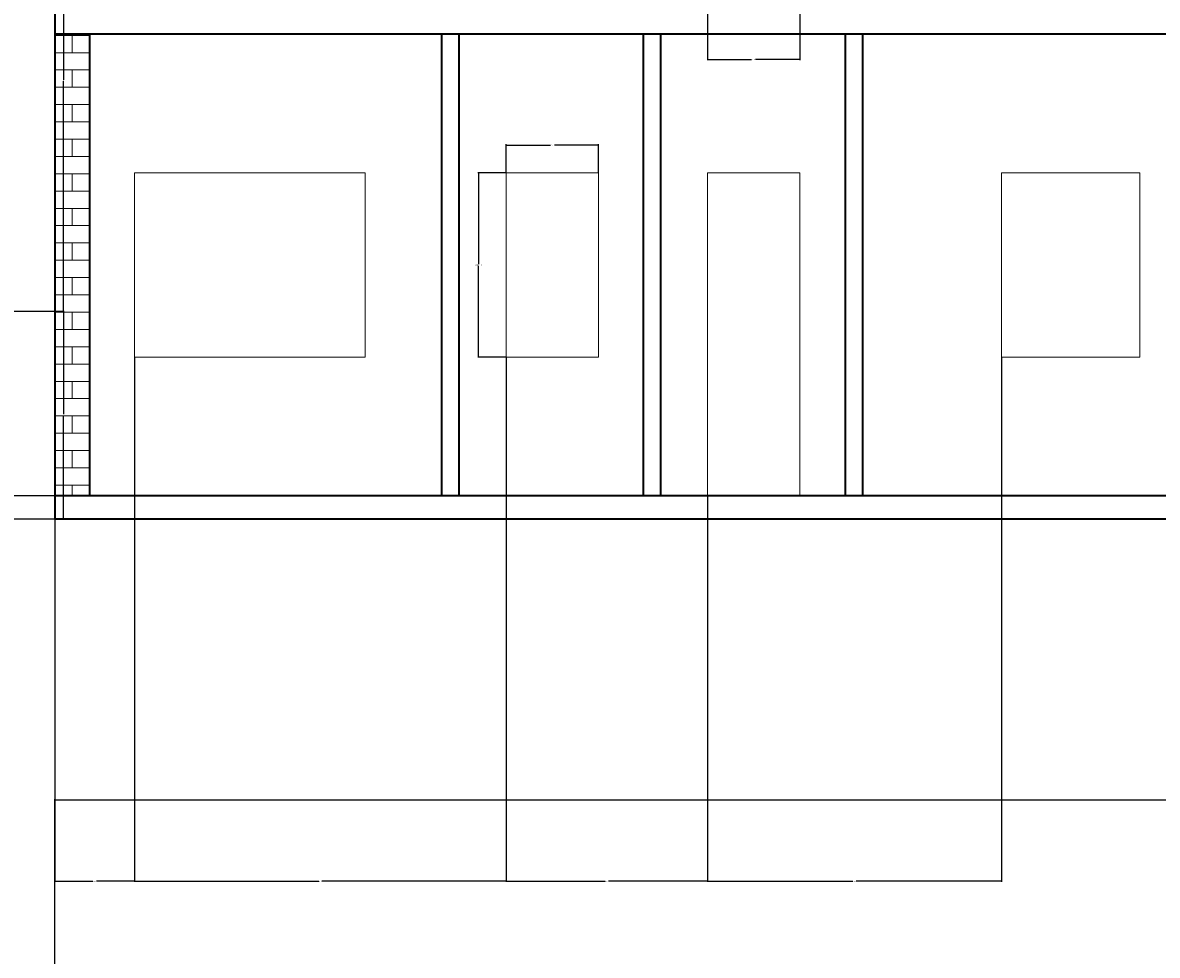
# Model space of a CAD drawing. Units: inches. Extents: x 2120 to 4013, y 1390 to 3019.
# Tile 55 of 59: x 3063 to 3358, y 2356 to 2598. Entities that reach past the tile are written whole.
import ezdxf

# ---------------------------------------------------------------- set-up
doc = ezdxf.new("R2010")
doc.units = ezdxf.units.IN
for name, color, linetype, lineweight in [('A-ANNO-DIMS', 2, 'Continuous', 18), ('A-DOOR', 3, 'Continuous', 18), ('A-GLAZ', 4, 'Continuous', 18), ('A-SECT', 7, 'Continuous', 35), ('A-WALL-PATT', 252, 'Continuous', 13)]:
    doc.layers.add(name, color=color, linetype=linetype, lineweight=lineweight)
doc.styles.get("Standard").update_dxf_attribs({"font": 'arial.ttf'})
doc.dimstyles.get("Standard").update_dxf_attribs({"dimtxt": 0.18, "dimasz": 0.18, "dimexe": 0.18, "dimexo": 0.0625, "dimgap": 0.09, "dimtad": 0, "dimtih": 1, "dimtoh": 1, "dimdec": 4, "dimzin": 0, "dimdsep": 46, "dimtxsty": 'Standard', "dimcen": 0.09, "dimadec": 0, "dimazin": 0, "dimtfac": 1, "dimtdec": 4, "dimtofl": 0, "dimtmove": 0, "dimatfit": 3, "dimfxl": 1, "dimtolj": 1, "dimtzin": 0, "dimarcsym": 0})

# ---------------------------------------------------------------- blocks, each defined once
blk = doc.blocks.new('WIN-SECT-60IN')
for p, q in [((0, 48), (0, 0)), ((60, 48), (0, 48)), ((60, 48), (60, 0)), ((60, 0), (0, 0))]:
    blk.add_line(p, q)
blk = doc.blocks.new('WIN-SECT-24IN')
for p, q in [((0, 48), (0, 0)), ((0, 48), (0, 0)), ((24, 48), (0, 48)), ((24, 48), (24, 0)), ((24, 0), (0, 0))]:
    blk.add_line(p, q)
blk = doc.blocks.new('DOOR-SECT-24IN')
for p, q in [((0, 84), (0, 0)), ((24, 84), (0, 84)), ((24, 84), (24, 0))]:
    blk.add_line(p, q)
blk = doc.blocks.new('WIN-SECT-36IN')
for p, q in [((0, 48), (0, 0)), ((36, 48), (0, 48)), ((36, 48), (36, 0)), ((36, 0), (0, 0))]:
    blk.add_line(p, q)
blk = doc.blocks.new('*D201')
at = {"layer": 'A-ANNO-DIMS', "color": 0, "lineweight": -2, "transparency": 16777216}
for p, q in [((3189.03, 2559.31), (3181.72, 2559.31)), ((3181.9, 2559.13), (3181.9, 2535.49)), ((3181.9, 2511.49), (3181.9, 2535.13)), ((3189.03, 2511.31), (3181.72, 2511.31))]:
    blk.add_line(p, q, dxfattribs=at)
at = {"layer": 'A-ANNO-DIMS', "color": 0, "transparency": 16777216}
for points in [[(3181.87, 2559.13), (3181.93, 2559.13), (3181.9, 2559.31)], [(3181.87, 2511.49), (3181.93, 2511.49), (3181.9, 2511.31)]]:
    blk.add_solid(points, dxfattribs=at)
at = {"layer": 'Defpoints', "color": 0, "transparency": 16777216}
for p in [(3181.9, 2559.31), (3189.1, 2559.31), (3189.1, 2511.31)]:
    blk.add_point(p, dxfattribs=at)
at = {"layer": 'A-ANNO-DIMS', "color": 0, "transparency": 16777216, "insert": (3181.9, 2535.31), "char_height": 0.18, "attachment_point": 5}
blk.add_mtext('\\A1;WINDOW 48 TYP.', dxfattribs=at)
blk = doc.blocks.new('*D202')
at = {"layer": 'A-ANNO-DIMS', "color": 0, "lineweight": -2, "transparency": 16777216}
for p, q in [((3189.1, 2559.37), (3189.1, 2566.69)), ((3189.28, 2566.51), (3200.57, 2566.51)), ((3212.92, 2566.51), (3201.63, 2566.51)), ((3213.1, 2559.37), (3213.1, 2566.69))]:
    blk.add_line(p, q, dxfattribs=at)
at = {"layer": 'A-ANNO-DIMS', "color": 0, "transparency": 16777216}
for points in [[(3189.28, 2566.54), (3189.28, 2566.48), (3189.1, 2566.51)], [(3212.92, 2566.54), (3212.92, 2566.48), (3213.1, 2566.51)]]:
    blk.add_solid(points, dxfattribs=at)
at = {"layer": 'Defpoints', "color": 0, "transparency": 16777216}
for p in [(3213.1, 2566.51), (3189.1, 2559.31), (3213.1, 2559.31)]:
    blk.add_point(p, dxfattribs=at)
at = {"layer": 'A-ANNO-DIMS', "color": 0, "transparency": 16777216, "insert": (3201.1, 2566.51), "char_height": 0.18, "attachment_point": 5}
blk.add_mtext('\\A1;24 TYP.', dxfattribs=at)
blk = doc.blocks.new('*D204')
at = {"layer": 'A-ANNO-DIMS', "color": 0, "lineweight": -2, "transparency": 16777216}
for p, q in [((3241.44, 2601.25), (3241.44, 2588.53)), ((3265.44, 2601.25), (3265.44, 2588.53)), ((3241.62, 2588.71), (3252.91, 2588.71)), ((3265.26, 2588.71), (3253.97, 2588.71))]:
    blk.add_line(p, q, dxfattribs=at)
at = {"layer": 'A-ANNO-DIMS', "color": 0, "transparency": 16777216}
for points in [[(3241.62, 2588.74), (3241.62, 2588.68), (3241.44, 2588.71)], [(3265.26, 2588.74), (3265.26, 2588.68), (3265.44, 2588.71)]]:
    blk.add_solid(points, dxfattribs=at)
at = {"layer": 'Defpoints', "color": 0, "transparency": 16777216}
for p in [(3241.44, 2601.31), (3265.44, 2601.31), (3265.44, 2588.71)]:
    blk.add_point(p, dxfattribs=at)
at = {"layer": 'A-ANNO-DIMS', "color": 0, "transparency": 16777216, "insert": (3253.44, 2588.71), "char_height": 0.18, "attachment_point": 5}
blk.add_mtext('\\A1;24 TYP.', dxfattribs=at)
blk = doc.blocks.new('*D216')
at = {"layer": 'A-ANNO-DIMS', "color": 0, "lineweight": -2, "transparency": 16777216}
for p, q in [((3071.73, 2352.59), (3071.73, 2396.46)), ((3071.91, 2396.28), (3444.95, 2396.28)), ((3818.55, 2396.28), (3445.52, 2396.28)), ((3818.73, 2352.59), (3818.73, 2396.46))]:
    blk.add_line(p, q, dxfattribs=at)
at = {"layer": 'A-ANNO-DIMS', "color": 0, "transparency": 16777216}
for points in [[(3071.91, 2396.31), (3071.91, 2396.25), (3071.73, 2396.28)], [(3818.55, 2396.31), (3818.55, 2396.25), (3818.73, 2396.28)]]:
    blk.add_solid(points, dxfattribs=at)
at = {"layer": 'Defpoints', "color": 0, "transparency": 16777216}
for p in [(3818.73, 2396.28), (3071.73, 2352.53), (3818.73, 2352.53)]:
    blk.add_point(p, dxfattribs=at)
at = {"layer": 'A-ANNO-DIMS', "color": 0, "transparency": 16777216, "insert": (3445.23, 2396.28), "char_height": 0.18, "attachment_point": 5}
blk.add_mtext('\\A1;747', dxfattribs=at)
blk = doc.blocks.new('*D233')
at = {"layer": 'A-ANNO-DIMS', "color": 0, "lineweight": -2, "transparency": 16777216}
for p, q in [((3009.8, 2523.31), (3074.11, 2523.31)), ((3073.93, 2523.13), (3073.93, 2496.49)), ((3073.93, 2469.49), (3073.93, 2496.13)), ((3009.8, 2469.31), (3074.11, 2469.31))]:
    blk.add_line(p, q, dxfattribs=at)
at = {"layer": 'A-ANNO-DIMS', "color": 0, "transparency": 16777216}
for points in [[(3073.9, 2523.13), (3073.96, 2523.13), (3073.93, 2523.31)], [(3073.9, 2469.49), (3073.96, 2469.49), (3073.93, 2469.31)]]:
    blk.add_solid(points, dxfattribs=at)
at = {"layer": 'Defpoints', "color": 0, "transparency": 16777216}
for p in [(3009.73, 2523.31), (3073.93, 2523.31), (3009.73, 2469.31)]:
    blk.add_point(p, dxfattribs=at)
at = {"layer": 'A-ANNO-DIMS', "color": 0, "transparency": 16777216, "insert": (3073.93, 2496.31), "char_height": 0.18, "attachment_point": 5}
blk.add_mtext('\\A1;54', dxfattribs=at)
blk = doc.blocks.new('*D234')
at = {"layer": 'A-ANNO-DIMS', "color": 0, "lineweight": -2, "transparency": 16777216}
for p, q in [((3033.8, 2643.31), (3074.11, 2643.31)), ((3073.93, 2643.13), (3073.93, 2583.49)), ((3073.93, 2523.49), (3073.93, 2583.13)), ((3009.8, 2523.31), (3074.11, 2523.31))]:
    blk.add_line(p, q, dxfattribs=at)
at = {"layer": 'A-ANNO-DIMS', "color": 0, "transparency": 16777216}
for points in [[(3073.9, 2643.13), (3073.96, 2643.13), (3073.93, 2643.31)], [(3073.9, 2523.49), (3073.96, 2523.49), (3073.93, 2523.31)]]:
    blk.add_solid(points, dxfattribs=at)
at = {"layer": 'Defpoints', "color": 0, "transparency": 16777216}
for p in [(3033.73, 2643.31), (3073.93, 2643.31), (3009.73, 2523.31)]:
    blk.add_point(p, dxfattribs=at)
at = {"layer": 'A-ANNO-DIMS', "color": 0, "transparency": 16777216, "insert": (3073.93, 2583.31), "char_height": 0.18, "attachment_point": 5}
blk.add_mtext('\\A1;120', dxfattribs=at)
blk = doc.blocks.new('*D238')
at = {"layer": 'A-ANNO-DIMS', "color": 0, "lineweight": -2, "transparency": 16777216}
for p, q in [((3071.67, 2601.31), (3026.6, 2601.31)), ((3026.78, 2601.13), (3026.78, 2538.49)), ((3026.78, 2475.49), (3026.78, 2538.13)), ((3071.67, 2475.31), (3026.6, 2475.31))]:
    blk.add_line(p, q, dxfattribs=at)
at = {"layer": 'A-ANNO-DIMS', "color": 0, "transparency": 16777216}
for points in [[(3026.75, 2601.13), (3026.81, 2601.13), (3026.78, 2601.31)], [(3026.75, 2475.49), (3026.81, 2475.49), (3026.78, 2475.31)]]:
    blk.add_solid(points, dxfattribs=at)
at = {"layer": 'Defpoints', "color": 0, "transparency": 16777216}
for p in [(3026.78, 2601.31), (3071.73, 2601.31), (3071.73, 2475.31)]:
    blk.add_point(p, dxfattribs=at)
at = {"layer": 'A-ANNO-DIMS', "color": 0, "transparency": 16777216, "insert": (3026.78, 2538.31), "char_height": 0.18, "attachment_point": 5}
blk.add_mtext('\\A1;126', dxfattribs=at)
blk = doc.blocks.new('*D241')
at = {"layer": 'A-ANNO-DIMS', "color": 0, "lineweight": -2, "transparency": 16777216}
for p, q in [((3092.38, 2511.25), (3092.38, 2374.91)), ((3071.73, 2475.25), (3071.73, 2374.91)), ((3071.91, 2375.09), (3081.59, 2375.09)), ((3092.2, 2375.09), (3082.52, 2375.09))]:
    blk.add_line(p, q, dxfattribs=at)
at = {"layer": 'A-ANNO-DIMS', "color": 0, "transparency": 16777216}
for points in [[(3071.91, 2375.12), (3071.91, 2375.06), (3071.73, 2375.09)], [(3092.2, 2375.12), (3092.2, 2375.06), (3092.38, 2375.09)]]:
    blk.add_solid(points, dxfattribs=at)
at = {"layer": 'Defpoints', "color": 0, "transparency": 16777216}
for p in [(3092.38, 2511.31), (3071.73, 2475.31), (3092.38, 2375.09)]:
    blk.add_point(p, dxfattribs=at)
at = {"layer": 'A-ANNO-DIMS', "color": 0, "transparency": 16777216, "insert": (3082.06, 2375.09), "char_height": 0.18, "attachment_point": 5}
blk.add_mtext('\\A1;20.646', dxfattribs=at)
blk = doc.blocks.new('*D242')
at = {"layer": 'A-ANNO-DIMS', "color": 0, "lineweight": -2, "transparency": 16777216}
for p, q in [((3092.38, 2511.25), (3092.38, 2374.91)), ((3189.1, 2511.25), (3189.1, 2374.91)), ((3092.56, 2375.09), (3140.35, 2375.09)), ((3188.92, 2375.09), (3141.13, 2375.09))]:
    blk.add_line(p, q, dxfattribs=at)
at = {"layer": 'A-ANNO-DIMS', "color": 0, "transparency": 16777216}
for points in [[(3092.56, 2375.12), (3092.56, 2375.06), (3092.38, 2375.09)], [(3188.92, 2375.12), (3188.92, 2375.06), (3189.1, 2375.09)]]:
    blk.add_solid(points, dxfattribs=at)
at = {"layer": 'Defpoints', "color": 0, "transparency": 16777216}
for p in [(3092.38, 2511.31), (3189.1, 2511.31), (3189.1, 2375.09)]:
    blk.add_point(p, dxfattribs=at)
at = {"layer": 'A-ANNO-DIMS', "color": 0, "transparency": 16777216, "insert": (3140.74, 2375.09), "char_height": 0.18, "attachment_point": 5}
blk.add_mtext('\\A1;96.72', dxfattribs=at)
blk = doc.blocks.new('*D243')
at = {"layer": 'A-ANNO-DIMS', "color": 0, "lineweight": -2, "transparency": 16777216}
for p, q in [((3189.1, 2511.25), (3189.1, 2374.91)), ((3241.44, 2475.25), (3241.44, 2374.91)), ((3189.28, 2375.09), (3214.87, 2375.09)), ((3241.26, 2375.09), (3215.66, 2375.09))]:
    blk.add_line(p, q, dxfattribs=at)
at = {"layer": 'A-ANNO-DIMS', "color": 0, "transparency": 16777216}
for points in [[(3189.28, 2375.12), (3189.28, 2375.06), (3189.1, 2375.09)], [(3241.26, 2375.12), (3241.26, 2375.06), (3241.44, 2375.09)]]:
    blk.add_solid(points, dxfattribs=at)
at = {"layer": 'Defpoints', "color": 0, "transparency": 16777216}
for p in [(3189.1, 2511.31), (3241.44, 2475.31), (3241.44, 2375.09)]:
    blk.add_point(p, dxfattribs=at)
at = {"layer": 'A-ANNO-DIMS', "color": 0, "transparency": 16777216, "insert": (3215.27, 2375.09), "char_height": 0.18, "attachment_point": 5}
blk.add_mtext('\\A1;52.34', dxfattribs=at)
blk = doc.blocks.new('*D244')
at = {"layer": 'A-ANNO-DIMS', "color": 0, "lineweight": -2, "transparency": 16777216}
for p, q in [((3317.91, 2511.25), (3317.91, 2374.91)), ((3241.44, 2475.25), (3241.44, 2374.91)), ((3241.62, 2375.09), (3279.28, 2375.09)), ((3317.73, 2375.09), (3280.07, 2375.09))]:
    blk.add_line(p, q, dxfattribs=at)
at = {"layer": 'A-ANNO-DIMS', "color": 0, "transparency": 16777216}
for points in [[(3241.62, 2375.12), (3241.62, 2375.06), (3241.44, 2375.09)], [(3317.73, 2375.12), (3317.73, 2375.06), (3317.91, 2375.09)]]:
    blk.add_solid(points, dxfattribs=at)
at = {"layer": 'Defpoints', "color": 0, "transparency": 16777216}
for p in [(3317.91, 2511.31), (3241.44, 2475.31), (3317.91, 2375.09)]:
    blk.add_point(p, dxfattribs=at)
at = {"layer": 'A-ANNO-DIMS', "color": 0, "transparency": 16777216, "insert": (3279.67, 2375.09), "char_height": 0.18, "attachment_point": 5}
blk.add_mtext('\\A1;76.48', dxfattribs=at)

msp = doc.modelspace()

# ---------------------------------------------------------------- hatches: boundary and pattern name
at = {"layer": 'A-WALL-PATT'}
h = msp.add_hatch(dxfattribs=at)
h.set_pattern_fill('ANSI32', color=256)
h.paths.add_polyline_path([(2271.7331, 2343.531), (2283.3788, 2343.531), (2283.3788, 2348.031), (2283.3788, 2352.5306), (2262.7331, 2352.5306), (2262.7331, 2182.638), (2267.2331, 2182.638), (2271.7331, 2182.638), (2271.7331, 2219.031), (2391.7331, 2219.031), (2391.7331, 2214.189), (2393.9831, 2214.189), (2396.2331, 2214.189), (2396.2331, 2219.031), (2420.2331, 2219.031), (2420.2331, 2225.7535), (2417.2197, 2225.7535), (2415.7331, 2225.7535), (2415.7331, 2223.5306), (2271.7331, 2223.5306)])
h.paths.add_polyline_path([(2380.0942, 2352.5306), (2343.3788, 2352.5306), (2343.3788, 2343.531), (2363.2331, 2343.531), (2363.2331, 2288.8489), (2365.4831, 2288.8489), (2367.7331, 2288.8489), (2367.7331, 2343.531), (2380.0942, 2343.531)], flags=17)
h.paths.add_polyline_path([(2432.4339, 2352.5306), (2404.0943, 2352.5306), (2404.0943, 2343.531), (2415.7331, 2343.531), (2415.7331, 2264.0306), (2367.7331, 2264.0306), (2367.7331, 2266.4872), (2363.2331, 2266.4872), (2363.2331, 2259.531), (2367.7331, 2259.531), (2415.7331, 2259.531), (2415.7331, 2255.0658), (2420.2331, 2255.0658), (2420.2331, 2259.531), (2424.5717, 2259.531), (2424.5717, 2261.781), (2424.5717, 2264.0306), (2420.2331, 2264.0306), (2420.2331, 2343.531), (2432.4339, 2343.531)])
h.paths.add_polyline_path([(2508.9115, 2352.5306), (2456.4339, 2352.5306), (2456.4339, 2343.531), (2468.2331, 2343.531), (2468.2331, 2264.0306), (2448.0487, 2264.0306), (2448.0487, 2259.531), (2468.2331, 2259.531), (2468.2331, 2255.5496), (2472.7331, 2255.5496), (2472.7331, 2343.531), (2508.9115, 2343.531)])
h.paths.add_polyline_path([(2637.7331, 2352.5306), (2544.9116, 2352.5306), (2544.9116, 2343.531), (2589.7331, 2343.531), (2633.2331, 2343.531), (2637.7331, 2343.531)])
h.paths.add_polyline_path([(2594.2331, 2343.5306), (2589.7331, 2343.5306), (2589.7331, 2259.5306), (2589.7331, 2252.4915), (2591.9831, 2252.4915), (2594.2331, 2252.4915)])
h.paths.add_polyline_path([(2637.7331, 2223.5306), (2594.2331, 2223.5306), (2594.2331, 2230.1988), (2591.9831, 2230.1988), (2589.7331, 2230.1988), (2589.7331, 2223.5306), (2472.7331, 2223.5306), (2468.2331, 2223.5306), (2468.2331, 2219.031), (2628.7331, 2219.031), (2628.7331, 2138.031), (2637.7331, 2138.031)])
h.paths.add_polyline_path([(3822.6535, 2458.4402), (3874.9468, 2458.4402), (3874.9468, 2476.9866), (3822.6535, 2476.9866)], flags=9)
h.paths.add_polyline_path([(3834.6921, 2781.8174), (3935.9206, 2781.8174), (3935.9206, 2800.3638), (3834.6921, 2800.3638)], flags=9)
h.paths.add_polyline_path([(3832.2843, 2837.9683), (3884.5776, 2837.9683), (3884.5776, 2856.5146), (3832.2843, 2856.5146)], flags=9)
h.paths.add_polyline_path([(3830.9388, 2861.4782), (3956.8958, 2861.4782), (3956.8958, 2880.0245), (3830.9388, 2880.0245)], flags=9)
h.paths.add_polyline_path([(3870.6966, 2352.5752), (3887.9272, 2352.5752), (3887.9272, 2377.3037), (3870.6966, 2377.3037)], flags=9)
h.paths.add_polyline_path([(3289.2701, 2413.161), (3435.2223, 2413.161), (3435.2223, 2450.2538), (3289.2701, 2450.2538)], flags=9)
h.paths.add_polyline_path([(2487.6944, 2414.3601), (2637.8335, 2414.3601), (2637.8335, 2451.4528), (2487.6944, 2451.4528)], flags=9)
h.paths.add_polyline_path([(2567.3724, 1457.9199), (2815.296, 1457.9199), (2815.296, 1495.0127), (2567.3724, 1495.0127)], flags=9)
h.paths.add_polyline_path([(2655.3825, 2093.2363), (2685.9555, 2093.2363), (2685.9555, 2111.8937), (2655.3825, 2111.8937)], flags=9)
h.paths.add_polyline_path([(2543.9218, 1550.6671), (2587.8406, 1550.6671), (2587.8406, 1569.3244), (2543.9218, 1569.3244)], flags=9)
h.paths.add_polyline_path([(2905.1384, 1543.8113), (2949.0572, 1543.8113), (2949.0572, 1562.4686), (2905.1384, 1562.4686)], flags=9)
h.paths.add_polyline_path([(2736.4118, 1702.4736), (2784.2153, 1702.4736), (2784.2153, 1721.1309), (2736.4118, 1721.1309)], flags=9)
h.paths.add_polyline_path([(2912.8666, 1710.4168), (2951.707, 1710.4168), (2951.707, 1729.0741), (2912.8666, 1729.0741)], flags=9)
h.paths.add_polyline_path([(2923.5785, 1763.5038), (2959.7279, 1763.5038), (2959.7279, 1782.1611), (2923.5785, 1782.1611)], flags=9)
h.paths.add_polyline_path([(2925.2114, 1809.6137), (2967.1861, 1809.6137), (2967.1861, 1828.271), (2925.2114, 1828.271)], flags=9)
h.paths.add_polyline_path([(2996.2711, 1878.9003), (2996.2711, 1913.109), (2977.6138, 1913.109), (2977.6138, 1878.9003)], flags=9)
h.paths.add_polyline_path([(2883.0859, 1895.7192), (2927.1855, 1895.7192), (2927.1855, 1914.3766), (2883.0859, 1914.3766)], flags=9)
h.paths.add_polyline_path([(2787.3924, 1810.8013), (2841.0213, 1810.8013), (2841.0213, 1829.4587), (2787.3924, 1829.4587)], flags=9)
h.paths.add_polyline_path([(2775.6399, 2101.7395), (2829.2689, 2101.7395), (2829.2689, 2120.3968), (2775.6399, 2120.3968)], flags=9)
h.paths.add_polyline_path([(2913.0263, 2075.817), (2951.8667, 2075.817), (2951.8667, 2094.4744), (2913.0263, 2094.4744)], flags=9)
h.paths.add_polyline_path([(2929.966, 2133.3669), (2966.1154, 2133.3669), (2966.1154, 2152.0243), (2929.966, 2152.0243)], flags=9)
h.paths.add_polyline_path([(2932.7502, 2182.6088), (2968.8996, 2182.6088), (2968.8996, 2201.2662), (2932.7502, 2201.2662)], flags=9)
h.paths.add_polyline_path([(2996.0681, 2266.3173), (2996.0681, 2300.5261), (2977.4108, 2300.5261), (2977.4108, 2266.3173)], flags=9)
h.paths.add_polyline_path([(2885.1039, 2279.2186), (2929.2035, 2279.2186), (2929.2035, 2297.8759), (2885.1039, 2297.8759)], flags=9)
h.paths.add_polyline_path([(2735.7042, 2218.3197), (2783.5078, 2218.3197), (2783.5078, 2236.9771), (2735.7042, 2236.9771)], flags=9)
h.paths.add_polyline_path([(2635.6049, 2044.0085), (2648.9678, 2044.0085), (2648.9678, 2054.312), (2635.6049, 2054.312)], flags=9)
h.paths.add_polyline_path([(2714.0148, 1923.0473), (2727.3777, 1923.0473), (2727.3777, 1933.3508), (2714.0148, 1933.3508)], flags=9)
h.paths.add_polyline_path([(2709.0345, 1988.1628), (2722.3974, 1988.1628), (2722.3974, 1998.4663), (2709.0345, 1998.4663)], flags=9)
h.paths.add_polyline_path([(2592.8935, 1962.1763), (2606.2564, 1962.1763), (2606.2564, 1972.4799), (2592.8935, 1972.4799)], flags=9)
h.paths.add_polyline_path([(2618.3996, 1985.9724), (2644.1942, 1985.9724), (2644.1942, 1996.2759), (2618.3996, 1996.2759)], flags=9)
h.paths.add_polyline_path([(2601.279, 1920.5869), (2614.6419, 1920.5869), (2614.6419, 1930.8904), (2601.279, 1930.8904)], flags=9)
h.paths.add_polyline_path([(2692.3278, 1932.7645), (2704.5311, 1932.7645), (2704.5311, 1943.0681), (2692.3278, 1943.0681)], flags=9)
h.paths.add_polyline_path([(2311.122, 1672.7318), (2355.0408, 1672.7318), (2355.0408, 1691.3892), (2311.122, 1691.3892)], flags=9)
h.paths.add_polyline_path([(2456.2551, 1632.3198), (2492.4796, 1632.3198), (2492.4796, 1650.9772), (2456.2551, 1650.9772)], flags=9)
h.paths.add_polyline_path([(2401.0766, 1631.4793), (2437.301, 1631.4793), (2437.301, 1650.1367), (2401.0766, 1650.1367)], flags=9)
h.paths.add_polyline_path([(2546.7054, 1700.9235), (2594.509, 1700.9235), (2594.509, 1719.5809), (2546.7054, 1719.5809)], flags=9)
h.paths.add_polyline_path([(2445.4866, 1766.9937), (2497.5261, 1766.9937), (2497.5261, 1785.651), (2445.4866, 1785.651)], flags=9)
h.paths.add_polyline_path([(2287.9992, 1739.7675), (2326.8396, 1739.7675), (2326.8396, 1758.4248), (2287.9992, 1758.4248)], flags=9)
h.paths.add_polyline_path([(2458.5279, 1924.7607), (2510.5675, 1924.7607), (2510.5675, 1943.4181), (2458.5279, 1943.4181)], flags=9)
h.paths.add_polyline_path([(2309.2811, 1902.7642), (2345.4305, 1902.7642), (2345.4305, 1921.4215), (2309.2811, 1921.4215)], flags=9)
h.paths.add_polyline_path([(2490.7554, 2018.9392), (2530.7896, 2018.9392), (2530.7896, 2037.5965), (2490.7554, 2037.5965)], flags=9)
h.paths.add_polyline_path([(2402.143, 2024.7393), (2438.5414, 2024.7393), (2438.5414, 2043.3966), (2402.143, 2043.3966)], flags=9)
h.paths.add_polyline_path([(2287.856, 1931.7926), (2326.6964, 1931.7926), (2326.6964, 1950.4499), (2287.856, 1950.4499)], flags=9)
h.paths.add_polyline_path([(2281.7979, 2193.5771), (2320.6383, 2193.5771), (2320.6383, 2212.2344), (2281.7979, 2212.2344)], flags=25)
h.paths.add_polyline_path([(2484.0754, 2093.892), (2536.115, 2093.892), (2536.115, 2112.5494), (2484.0754, 2112.5494)], flags=9)
h.paths.add_polyline_path([(2624.7948, 2281.8639), (2624.7948, 2311.4137), (2606.1375, 2311.4137), (2606.1375, 2281.8639)], flags=9)
h.paths.add_polyline_path([(2507.5036, 2290.3639), (2541.934, 2290.3639), (2541.934, 2309.0212), (2507.5036, 2309.0212)], flags=9)
h.paths.add_polyline_path([(2423.1076, 2285.2202), (2459.332, 2285.2202), (2459.332, 2303.8776), (2423.1076, 2303.8776)], flags=9)
h.paths.add_polyline_path([(2374.5467, 2289.6272), (2410.7711, 2289.6272), (2410.7711, 2308.2846), (2374.5467, 2308.2846)], flags=25)
h.paths.add_polyline_path([(2277.4907, 2227.5651), (2316.3311, 2227.5651), (2316.3311, 2246.2224), (2277.4907, 2246.2224)], flags=25)
h.paths.add_polyline_path([(2655.3825, 2093.2367), (2685.9555, 2093.2367), (2685.9555, 2111.894), (2655.3825, 2111.894)], flags=9)
h.paths.add_polyline_path([(2543.9217, 1550.6674), (2587.8406, 1550.6674), (2587.8406, 1569.3247), (2543.9217, 1569.3247)], flags=9)
h.paths.add_polyline_path([(2905.1384, 1543.8116), (2949.0572, 1543.8116), (2949.0572, 1562.4689), (2905.1384, 1562.4689)], flags=9)
h.paths.add_polyline_path([(2736.4118, 1702.4739), (2784.2153, 1702.4739), (2784.2153, 1721.1312), (2736.4118, 1721.1312)], flags=9)
h.paths.add_polyline_path([(2912.8666, 1710.4171), (2951.707, 1710.4171), (2951.707, 1729.0744), (2912.8666, 1729.0744)], flags=9)
h.paths.add_polyline_path([(2923.5785, 1763.5041), (2959.7279, 1763.5041), (2959.7279, 1782.1614), (2923.5785, 1782.1614)], flags=9)
h.paths.add_polyline_path([(2925.2114, 1809.614), (2967.1861, 1809.614), (2967.1861, 1828.2713), (2925.2114, 1828.2713)], flags=9)
h.paths.add_polyline_path([(2996.2711, 1878.9006), (2996.2711, 1913.1094), (2977.6137, 1913.1094), (2977.6137, 1878.9006)], flags=9)
h.paths.add_polyline_path([(2883.0859, 1895.7195), (2927.1855, 1895.7195), (2927.1855, 1914.3769), (2883.0859, 1914.3769)], flags=9)
h.paths.add_polyline_path([(2787.3924, 1810.8016), (2841.0213, 1810.8016), (2841.0213, 1829.459), (2787.3924, 1829.459)], flags=9)
h.paths.add_polyline_path([(2775.6399, 2101.7398), (2829.2688, 2101.7398), (2829.2688, 2120.3971), (2775.6399, 2120.3971)], flags=9)
h.paths.add_polyline_path([(2913.0263, 2075.8173), (2951.8667, 2075.8173), (2951.8667, 2094.4747), (2913.0263, 2094.4747)], flags=9)
h.paths.add_polyline_path([(2929.966, 2133.3672), (2966.1154, 2133.3672), (2966.1154, 2152.0246), (2929.966, 2152.0246)], flags=9)
h.paths.add_polyline_path([(2932.7502, 2182.6091), (2968.8996, 2182.6091), (2968.8996, 2201.2665), (2932.7502, 2201.2665)], flags=9)
h.paths.add_polyline_path([(2996.0681, 2266.3176), (2996.0681, 2300.5264), (2977.4108, 2300.5264), (2977.4108, 2266.3176)], flags=9)
h.paths.add_polyline_path([(2885.1039, 2279.2189), (2929.2035, 2279.2189), (2929.2035, 2297.8762), (2885.1039, 2297.8762)], flags=9)
h.paths.add_polyline_path([(2735.7042, 2218.32), (2783.5078, 2218.32), (2783.5078, 2236.9774), (2735.7042, 2236.9774)], flags=9)
h.paths.add_polyline_path([(2635.6048, 2044.0088), (2648.9677, 2044.0088), (2648.9677, 2054.3123), (2635.6048, 2054.3123)], flags=9)
h.paths.add_polyline_path([(2714.0148, 1923.0476), (2727.3777, 1923.0476), (2727.3777, 1933.3511), (2714.0148, 1933.3511)], flags=9)
h.paths.add_polyline_path([(2709.0345, 1988.1631), (2722.3974, 1988.1631), (2722.3974, 1998.4666), (2709.0345, 1998.4666)], flags=9)
h.paths.add_polyline_path([(2592.8935, 1962.1766), (2606.2564, 1962.1766), (2606.2564, 1972.4802), (2592.8935, 1972.4802)], flags=9)
h.paths.add_polyline_path([(2618.3995, 1985.9727), (2644.1942, 1985.9727), (2644.1942, 1996.2762), (2618.3995, 1996.2762)], flags=9)
h.paths.add_polyline_path([(2601.279, 1920.5872), (2614.6419, 1920.5872), (2614.6419, 1930.8908), (2601.279, 1930.8908)], flags=9)
h.paths.add_polyline_path([(2692.3278, 1932.7648), (2704.5311, 1932.7648), (2704.5311, 1943.0684), (2692.3278, 1943.0684)], flags=9)
h.paths.add_polyline_path([(2311.122, 1672.7321), (2355.0408, 1672.7321), (2355.0408, 1691.3895), (2311.122, 1691.3895)], flags=9)
h.paths.add_polyline_path([(2456.2551, 1632.3201), (2492.4795, 1632.3201), (2492.4795, 1650.9775), (2456.2551, 1650.9775)], flags=9)
h.paths.add_polyline_path([(2401.0766, 1631.4796), (2437.301, 1631.4796), (2437.301, 1650.137), (2401.0766, 1650.137)], flags=9)
h.paths.add_polyline_path([(2546.7054, 1700.9238), (2594.509, 1700.9238), (2594.509, 1719.5812), (2546.7054, 1719.5812)], flags=9)
h.paths.add_polyline_path([(2445.4866, 1766.994), (2497.5261, 1766.994), (2497.5261, 1785.6513), (2445.4866, 1785.6513)], flags=9)
h.paths.add_polyline_path([(2287.9992, 1739.7678), (2326.8396, 1739.7678), (2326.8396, 1758.4251), (2287.9992, 1758.4251)], flags=9)
h.paths.add_polyline_path([(2458.5279, 1924.7611), (2510.5675, 1924.7611), (2510.5675, 1943.4184), (2458.5279, 1943.4184)], flags=9)
h.paths.add_polyline_path([(2309.2811, 1902.7645), (2345.4305, 1902.7645), (2345.4305, 1921.4218), (2309.2811, 1921.4218)], flags=9)
h.paths.add_polyline_path([(2490.7554, 2018.9395), (2530.7895, 2018.9395), (2530.7895, 2037.5968), (2490.7554, 2037.5968)], flags=9)
h.paths.add_polyline_path([(2402.143, 2024.7396), (2438.5413, 2024.7396), (2438.5413, 2043.3969), (2402.143, 2043.3969)], flags=9)
h.paths.add_polyline_path([(2287.856, 1931.7929), (2326.6964, 1931.7929), (2326.6964, 1950.4502), (2287.856, 1950.4502)], flags=9)
h.paths.add_polyline_path([(2281.7979, 2193.5774), (2320.6383, 2193.5774), (2320.6383, 2212.2347), (2281.7979, 2212.2347)], flags=25)
h.paths.add_polyline_path([(2484.0754, 2093.8924), (2536.115, 2093.8924), (2536.115, 2112.5497), (2484.0754, 2112.5497)], flags=9)
h.paths.add_polyline_path([(2624.7948, 2281.8642), (2624.7948, 2311.414), (2606.1374, 2311.414), (2606.1374, 2281.8642)], flags=9)
h.paths.add_polyline_path([(2507.5035, 2290.3642), (2541.934, 2290.3642), (2541.934, 2309.0215), (2507.5035, 2309.0215)], flags=9)
h.paths.add_polyline_path([(2423.1075, 2285.2205), (2459.332, 2285.2205), (2459.332, 2303.8779), (2423.1075, 2303.8779)], flags=9)
h.paths.add_polyline_path([(2374.5467, 2289.6275), (2410.7711, 2289.6275), (2410.7711, 2308.2849), (2374.5467, 2308.2849)], flags=25)
h.paths.add_polyline_path([(2277.4907, 2227.5654), (2316.3311, 2227.5654), (2316.3311, 2246.2227), (2277.4907, 2246.2227)], flags=25)
h = msp.add_hatch(dxfattribs=at)
h.set_pattern_fill('ANSI32', color=256)
h.paths.add_polyline_path([(2271.7331, 1980.389), (2262.7331, 1980.389), (2262.7331, 1912.8434), (2267.2331, 1912.8434), (2271.7331, 1912.8434), (2271.7331, 1922.531), (2351.2331, 1922.531), (2351.2331, 1901.4728), (2355.7331, 1901.4728), (2355.7331, 1922.531), (2357.9815, 1922.531), (2357.9815, 1926.5306), (2271.7331, 1926.5306)])
h.paths.add_polyline_path([(2589.2331, 1949.1622), (2584.7331, 1949.1622), (2580.2331, 1949.1622), (2580.2331, 1874.5306), (2355.7331, 1874.5306), (2355.7331, 1880.1922), (2351.2331, 1880.1922), (2351.2331, 1874.5306), (2271.7331, 1874.5306), (2271.7331, 1888.8431), (2262.7331, 1888.8431), (2262.7331, 1842.2909), (2267.2331, 1842.2909), (2271.7331, 1842.2909), (2271.7331, 1865.531), (2415.7331, 1865.531), (2415.7331, 1779.7286), (2420.2331, 1779.7286), (2420.2331, 1865.531), (2589.2331, 1865.531)])
h.paths.add_polyline_path([(2271.7331, 1782.2906), (2262.7331, 1782.2906), (2262.7331, 1711.4639), (2267.2331, 1711.4639), (2271.7331, 1711.4639), (2271.7331, 1738.031), (2420.2331, 1738.031), (2420.2331, 1742.531), (2420.2331, 1747.3376), (2417.9831, 1747.3376), (2415.7331, 1747.3376), (2415.7331, 1742.5306), (2271.7331, 1742.5306)])
h.paths.add_polyline_path([(2271.7331, 1627.031), (2362.3957, 1627.031), (2362.3957, 1629.281), (2362.3957, 1631.5306), (2271.7331, 1631.5306), (2271.7331, 1675.4636), (2262.7331, 1675.4636), (2262.7331, 1581.531), (2405.3032, 1581.531), (2405.3032, 1586.031), (2405.3032, 1590.5306), (2396.2331, 1590.5306), (2396.2331, 1691.4513), (2418.7206, 1691.4513), (2418.7206, 1695.951), (2396.2331, 1695.951), (2391.7331, 1695.951), (2391.7331, 1631.5306), (2386.7425, 1631.5306), (2386.7425, 1629.2806), (2386.7425, 1627.031), (2391.7331, 1627.031), (2391.7331, 1586.1709), (2271.7331, 1586.1709)])
h.paths.add_polyline_path([(2459.6703, 1590.5306), (2429.3032, 1590.5306), (2429.3032, 1581.531), (2459.6703, 1581.531), (2459.6703, 1586.031)])
h.paths.add_polyline_path([(2501.2331, 1590.531), (2501.2331, 1665.0195), (2498.9831, 1665.0195), (2496.7331, 1665.0195), (2496.7331, 1590.5306), (2483.8201, 1590.5306), (2483.8201, 1590.1579), (2483.6704, 1590.1579), (2483.6704, 1581.531), (2505.0196, 1581.531), (2505.0196, 1583.781), (2505.0196, 1586.0306), (2501.2331, 1586.0306)])
h.paths.add_polyline_path([(2544.1361, 1583.781), (2544.1361, 1586.0306), (2527.1368, 1586.0306), (2527.1368, 1583.7806), (2527.1368, 1581.531), (2544.1361, 1581.531)])
h.paths.add_polyline_path([(3822.6535, 2458.4402), (3874.9468, 2458.4402), (3874.9468, 2476.9866), (3822.6535, 2476.9866)], flags=9)
h.paths.add_polyline_path([(3834.6921, 2781.8174), (3935.9206, 2781.8174), (3935.9206, 2800.3638), (3834.6921, 2800.3638)], flags=9)
h.paths.add_polyline_path([(3832.2843, 2837.9683), (3884.5776, 2837.9683), (3884.5776, 2856.5146), (3832.2843, 2856.5146)], flags=9)
h.paths.add_polyline_path([(3830.9388, 2861.4782), (3956.8958, 2861.4782), (3956.8958, 2880.0245), (3830.9388, 2880.0245)], flags=9)
h.paths.add_polyline_path([(3870.6966, 2352.5752), (3887.9272, 2352.5752), (3887.9272, 2377.3037), (3870.6966, 2377.3037)], flags=9)
h.paths.add_polyline_path([(3289.2701, 2413.161), (3435.2223, 2413.161), (3435.2223, 2450.2538), (3289.2701, 2450.2538)], flags=9)
h.paths.add_polyline_path([(2487.6944, 2414.3601), (2637.8335, 2414.3601), (2637.8335, 2451.4528), (2487.6944, 2451.4528)], flags=9)
h.paths.add_polyline_path([(2567.3724, 1457.9199), (2815.296, 1457.9199), (2815.296, 1495.0127), (2567.3724, 1495.0127)], flags=9)
h.paths.add_polyline_path([(2655.3825, 2093.2363), (2685.9555, 2093.2363), (2685.9555, 2111.8937), (2655.3825, 2111.8937)], flags=9)
h.paths.add_polyline_path([(2543.9218, 1550.6671), (2587.8406, 1550.6671), (2587.8406, 1569.3244), (2543.9218, 1569.3244)], flags=9)
h.paths.add_polyline_path([(2905.1384, 1543.8113), (2949.0572, 1543.8113), (2949.0572, 1562.4686), (2905.1384, 1562.4686)], flags=9)
h.paths.add_polyline_path([(2736.4118, 1702.4736), (2784.2153, 1702.4736), (2784.2153, 1721.1309), (2736.4118, 1721.1309)], flags=9)
h.paths.add_polyline_path([(2912.8666, 1710.4168), (2951.707, 1710.4168), (2951.707, 1729.0741), (2912.8666, 1729.0741)], flags=9)
h.paths.add_polyline_path([(2923.5785, 1763.5038), (2959.7279, 1763.5038), (2959.7279, 1782.1611), (2923.5785, 1782.1611)], flags=9)
h.paths.add_polyline_path([(2925.2114, 1809.6137), (2967.1861, 1809.6137), (2967.1861, 1828.271), (2925.2114, 1828.271)], flags=9)
h.paths.add_polyline_path([(2996.2711, 1878.9003), (2996.2711, 1913.109), (2977.6138, 1913.109), (2977.6138, 1878.9003)], flags=9)
h.paths.add_polyline_path([(2883.0859, 1895.7192), (2927.1855, 1895.7192), (2927.1855, 1914.3766), (2883.0859, 1914.3766)], flags=9)
h.paths.add_polyline_path([(2787.3924, 1810.8013), (2841.0213, 1810.8013), (2841.0213, 1829.4587), (2787.3924, 1829.4587)], flags=9)
h.paths.add_polyline_path([(2775.6399, 2101.7395), (2829.2689, 2101.7395), (2829.2689, 2120.3968), (2775.6399, 2120.3968)], flags=9)
h.paths.add_polyline_path([(2913.0263, 2075.817), (2951.8667, 2075.817), (2951.8667, 2094.4744), (2913.0263, 2094.4744)], flags=9)
h.paths.add_polyline_path([(2929.966, 2133.3669), (2966.1154, 2133.3669), (2966.1154, 2152.0243), (2929.966, 2152.0243)], flags=9)
h.paths.add_polyline_path([(2932.7502, 2182.6088), (2968.8996, 2182.6088), (2968.8996, 2201.2662), (2932.7502, 2201.2662)], flags=9)
h.paths.add_polyline_path([(2996.0681, 2266.3173), (2996.0681, 2300.5261), (2977.4108, 2300.5261), (2977.4108, 2266.3173)], flags=9)
h.paths.add_polyline_path([(2885.1039, 2279.2186), (2929.2035, 2279.2186), (2929.2035, 2297.8759), (2885.1039, 2297.8759)], flags=9)
h.paths.add_polyline_path([(2735.7042, 2218.3197), (2783.5078, 2218.3197), (2783.5078, 2236.9771), (2735.7042, 2236.9771)], flags=9)
h.paths.add_polyline_path([(2635.6049, 2044.0085), (2648.9678, 2044.0085), (2648.9678, 2054.312), (2635.6049, 2054.312)], flags=9)
h.paths.add_polyline_path([(2714.0148, 1923.0473), (2727.3777, 1923.0473), (2727.3777, 1933.3508), (2714.0148, 1933.3508)], flags=9)
h.paths.add_polyline_path([(2709.0345, 1988.1628), (2722.3974, 1988.1628), (2722.3974, 1998.4663), (2709.0345, 1998.4663)], flags=9)
h.paths.add_polyline_path([(2592.8935, 1962.1763), (2606.2564, 1962.1763), (2606.2564, 1972.4799), (2592.8935, 1972.4799)], flags=9)
h.paths.add_polyline_path([(2618.3996, 1985.9724), (2644.1942, 1985.9724), (2644.1942, 1996.2759), (2618.3996, 1996.2759)], flags=9)
h.paths.add_polyline_path([(2601.279, 1920.5869), (2614.6419, 1920.5869), (2614.6419, 1930.8904), (2601.279, 1930.8904)], flags=9)
h.paths.add_polyline_path([(2692.3278, 1932.7645), (2704.5311, 1932.7645), (2704.5311, 1943.0681), (2692.3278, 1943.0681)], flags=9)
h.paths.add_polyline_path([(2311.122, 1672.7318), (2355.0408, 1672.7318), (2355.0408, 1691.3892), (2311.122, 1691.3892)], flags=25)
h.paths.add_polyline_path([(2456.2551, 1632.3198), (2492.4796, 1632.3198), (2492.4796, 1650.9772), (2456.2551, 1650.9772)], flags=9)
h.paths.add_polyline_path([(2401.0766, 1631.4793), (2437.301, 1631.4793), (2437.301, 1650.1367), (2401.0766, 1650.1367)], flags=9)
h.paths.add_polyline_path([(2546.7054, 1700.9235), (2594.509, 1700.9235), (2594.509, 1719.5809), (2546.7054, 1719.5809)], flags=9)
h.paths.add_polyline_path([(2445.4866, 1766.9937), (2497.5261, 1766.9937), (2497.5261, 1785.651), (2445.4866, 1785.651)], flags=9)
h.paths.add_polyline_path([(2287.9992, 1739.7675), (2326.8396, 1739.7675), (2326.8396, 1758.4248), (2287.9992, 1758.4248)], flags=24)
h.paths.add_polyline_path([(2458.5279, 1924.7607), (2510.5675, 1924.7607), (2510.5675, 1943.4181), (2458.5279, 1943.4181)], flags=25)
h.paths.add_polyline_path([(2309.2811, 1902.7642), (2345.4305, 1902.7642), (2345.4305, 1921.4215), (2309.2811, 1921.4215)], flags=25)
h.paths.add_polyline_path([(2490.7554, 2018.9392), (2530.7896, 2018.9392), (2530.7896, 2037.5965), (2490.7554, 2037.5965)], flags=9)
h.paths.add_polyline_path([(2402.143, 2024.7393), (2438.5414, 2024.7393), (2438.5414, 2043.3966), (2402.143, 2043.3966)], flags=9)
h.paths.add_polyline_path([(2287.856, 1931.7926), (2326.6964, 1931.7926), (2326.6964, 1950.4499), (2287.856, 1950.4499)], flags=25)
h.paths.add_polyline_path([(2281.7979, 2193.5771), (2320.6383, 2193.5771), (2320.6383, 2212.2344), (2281.7979, 2212.2344)], flags=9)
h.paths.add_polyline_path([(2484.0754, 2093.892), (2536.115, 2093.892), (2536.115, 2112.5494), (2484.0754, 2112.5494)], flags=9)
h.paths.add_polyline_path([(2624.7948, 2281.8639), (2624.7948, 2311.4137), (2606.1375, 2311.4137), (2606.1375, 2281.8639)], flags=9)
h.paths.add_polyline_path([(2507.5036, 2290.3639), (2541.934, 2290.3639), (2541.934, 2309.0212), (2507.5036, 2309.0212)], flags=9)
h.paths.add_polyline_path([(2423.1076, 2285.2202), (2459.332, 2285.2202), (2459.332, 2303.8776), (2423.1076, 2303.8776)], flags=9)
h.paths.add_polyline_path([(2374.5467, 2289.6272), (2410.7711, 2289.6272), (2410.7711, 2308.2846), (2374.5467, 2308.2846)], flags=9)
h.paths.add_polyline_path([(2277.4907, 2227.5651), (2316.3311, 2227.5651), (2316.3311, 2246.2224), (2277.4907, 2246.2224)], flags=9)
h.paths.add_polyline_path([(2655.3825, 2093.2367), (2685.9555, 2093.2367), (2685.9555, 2111.894), (2655.3825, 2111.894)], flags=9)
h.paths.add_polyline_path([(2543.9217, 1550.6674), (2587.8406, 1550.6674), (2587.8406, 1569.3247), (2543.9217, 1569.3247)], flags=9)
h.paths.add_polyline_path([(2905.1384, 1543.8116), (2949.0572, 1543.8116), (2949.0572, 1562.4689), (2905.1384, 1562.4689)], flags=9)
h.paths.add_polyline_path([(2736.4118, 1702.4739), (2784.2153, 1702.4739), (2784.2153, 1721.1312), (2736.4118, 1721.1312)], flags=9)
h.paths.add_polyline_path([(2912.8666, 1710.4171), (2951.707, 1710.4171), (2951.707, 1729.0744), (2912.8666, 1729.0744)], flags=9)
h.paths.add_polyline_path([(2923.5785, 1763.5041), (2959.7279, 1763.5041), (2959.7279, 1782.1614), (2923.5785, 1782.1614)], flags=9)
h.paths.add_polyline_path([(2925.2114, 1809.614), (2967.1861, 1809.614), (2967.1861, 1828.2713), (2925.2114, 1828.2713)], flags=9)
h.paths.add_polyline_path([(2996.2711, 1878.9006), (2996.2711, 1913.1094), (2977.6137, 1913.1094), (2977.6137, 1878.9006)], flags=9)
h.paths.add_polyline_path([(2883.0859, 1895.7195), (2927.1855, 1895.7195), (2927.1855, 1914.3769), (2883.0859, 1914.3769)], flags=9)
h.paths.add_polyline_path([(2787.3924, 1810.8016), (2841.0213, 1810.8016), (2841.0213, 1829.459), (2787.3924, 1829.459)], flags=9)
h.paths.add_polyline_path([(2775.6399, 2101.7398), (2829.2688, 2101.7398), (2829.2688, 2120.3971), (2775.6399, 2120.3971)], flags=9)
h.paths.add_polyline_path([(2913.0263, 2075.8173), (2951.8667, 2075.8173), (2951.8667, 2094.4747), (2913.0263, 2094.4747)], flags=9)
h.paths.add_polyline_path([(2929.966, 2133.3672), (2966.1154, 2133.3672), (2966.1154, 2152.0246), (2929.966, 2152.0246)], flags=9)
h.paths.add_polyline_path([(2932.7502, 2182.6091), (2968.8996, 2182.6091), (2968.8996, 2201.2665), (2932.7502, 2201.2665)], flags=9)
h.paths.add_polyline_path([(2996.0681, 2266.3176), (2996.0681, 2300.5264), (2977.4108, 2300.5264), (2977.4108, 2266.3176)], flags=9)
h.paths.add_polyline_path([(2885.1039, 2279.2189), (2929.2035, 2279.2189), (2929.2035, 2297.8762), (2885.1039, 2297.8762)], flags=9)
h.paths.add_polyline_path([(2735.7042, 2218.32), (2783.5078, 2218.32), (2783.5078, 2236.9774), (2735.7042, 2236.9774)], flags=9)
h.paths.add_polyline_path([(2635.6048, 2044.0088), (2648.9677, 2044.0088), (2648.9677, 2054.3123), (2635.6048, 2054.3123)], flags=9)
h.paths.add_polyline_path([(2714.0148, 1923.0476), (2727.3777, 1923.0476), (2727.3777, 1933.3511), (2714.0148, 1933.3511)], flags=9)
h.paths.add_polyline_path([(2709.0345, 1988.1631), (2722.3974, 1988.1631), (2722.3974, 1998.4666), (2709.0345, 1998.4666)], flags=9)
h.paths.add_polyline_path([(2592.8935, 1962.1766), (2606.2564, 1962.1766), (2606.2564, 1972.4802), (2592.8935, 1972.4802)], flags=9)
h.paths.add_polyline_path([(2618.3995, 1985.9727), (2644.1942, 1985.9727), (2644.1942, 1996.2762), (2618.3995, 1996.2762)], flags=9)
h.paths.add_polyline_path([(2601.279, 1920.5872), (2614.6419, 1920.5872), (2614.6419, 1930.8908), (2601.279, 1930.8908)], flags=9)
h.paths.add_polyline_path([(2692.3278, 1932.7648), (2704.5311, 1932.7648), (2704.5311, 1943.0684), (2692.3278, 1943.0684)], flags=9)
h.paths.add_polyline_path([(2311.122, 1672.7321), (2355.0408, 1672.7321), (2355.0408, 1691.3895), (2311.122, 1691.3895)], flags=25)
h.paths.add_polyline_path([(2456.2551, 1632.3201), (2492.4795, 1632.3201), (2492.4795, 1650.9775), (2456.2551, 1650.9775)], flags=9)
h.paths.add_polyline_path([(2401.0766, 1631.4796), (2437.301, 1631.4796), (2437.301, 1650.137), (2401.0766, 1650.137)], flags=9)
h.paths.add_polyline_path([(2546.7054, 1700.9238), (2594.509, 1700.9238), (2594.509, 1719.5812), (2546.7054, 1719.5812)], flags=9)
h.paths.add_polyline_path([(2445.4866, 1766.994), (2497.5261, 1766.994), (2497.5261, 1785.6513), (2445.4866, 1785.6513)], flags=9)
h.paths.add_polyline_path([(2287.9992, 1739.7678), (2326.8396, 1739.7678), (2326.8396, 1758.4251), (2287.9992, 1758.4251)], flags=24)
h.paths.add_polyline_path([(2458.5279, 1924.7611), (2510.5675, 1924.7611), (2510.5675, 1943.4184), (2458.5279, 1943.4184)], flags=25)
h.paths.add_polyline_path([(2309.2811, 1902.7645), (2345.4305, 1902.7645), (2345.4305, 1921.4218), (2309.2811, 1921.4218)], flags=25)
h.paths.add_polyline_path([(2490.7554, 2018.9395), (2530.7895, 2018.9395), (2530.7895, 2037.5968), (2490.7554, 2037.5968)], flags=9)
h.paths.add_polyline_path([(2402.143, 2024.7396), (2438.5413, 2024.7396), (2438.5413, 2043.3969), (2402.143, 2043.3969)], flags=9)
h.paths.add_polyline_path([(2287.856, 1931.7929), (2326.6964, 1931.7929), (2326.6964, 1950.4502), (2287.856, 1950.4502)], flags=25)
h.paths.add_polyline_path([(2281.7979, 2193.5774), (2320.6383, 2193.5774), (2320.6383, 2212.2347), (2281.7979, 2212.2347)], flags=9)
h.paths.add_polyline_path([(2484.0754, 2093.8924), (2536.115, 2093.8924), (2536.115, 2112.5497), (2484.0754, 2112.5497)], flags=9)
h.paths.add_polyline_path([(2624.7948, 2281.8642), (2624.7948, 2311.414), (2606.1374, 2311.414), (2606.1374, 2281.8642)], flags=9)
h.paths.add_polyline_path([(2507.5035, 2290.3642), (2541.934, 2290.3642), (2541.934, 2309.0215), (2507.5035, 2309.0215)], flags=9)
h.paths.add_polyline_path([(2423.1075, 2285.2205), (2459.332, 2285.2205), (2459.332, 2303.8779), (2423.1075, 2303.8779)], flags=9)
h.paths.add_polyline_path([(2374.5467, 2289.6275), (2410.7711, 2289.6275), (2410.7711, 2308.2849), (2374.5467, 2308.2849)], flags=9)
h.paths.add_polyline_path([(2277.4907, 2227.5654), (2316.3311, 2227.5654), (2316.3311, 2246.2227), (2277.4907, 2246.2227)], flags=9)
h = msp.add_hatch(dxfattribs=at)
h.set_pattern_fill('BRICK', color=256, scale=0.708254, style=0)
h.paths.add_polyline_path([(3071.7347, 2475.3118), (3080.7347, 2475.3118), (3080.7347, 2595.3118), (3071.7347, 2595.3118)])

# ---------------------------------------------------------------- linework, layer by layer
at = {"layer": 'A-SECT'}
for p, q in [((3071.7347, 2769.3118), (3071.7347, 2583.3118)), ((3071.7347, 2643.3118), (3071.7347, 2469.3118)), ((3446.7347, 2595.3118), (3071.7347, 2595.3118)), ((3080.7347, 2595.3118), (3080.7347, 2475.3118)), ((3172.2347, 2595.3118), (3172.2347, 2475.3118)), ((3176.7347, 2595.3118), (3176.7347, 2475.3118)), ((3224.7347, 2595.3118), (3224.7347, 2475.3118)), ((3224.7347, 2595.3118), (3224.7347, 2475.3118)), ((3229.2347, 2595.3118), (3229.2347, 2475.3118)), ((3277.2347, 2595.3118), (3277.2347, 2475.3118)), ((3281.7347, 2595.3118), (3281.7347, 2475.3118)), ((3818.7347, 2475.3118), (3071.7347, 2475.3118)), ((3071.7347, 2469.3118), (3818.7347, 2469.3118))]:
    msp.add_line(p, q, dxfattribs=at)

# ---------------------------------------------------------------- block references
at = {"layer": 'A-DOOR'}
msp.add_blockref('DOOR-SECT-24IN', (3241.4354, 2475.3118), dxfattribs=at)
at = {"layer": 'A-GLAZ'}
for name, p in [('WIN-SECT-60IN', (3092.3803, 2511.3118)), ('WIN-SECT-24IN', (3189.0958, 2511.3118)), ('WIN-SECT-36IN', (3317.9131, 2511.3118))]:
    msp.add_blockref(name, p, dxfattribs=at)

# ---------------------------------------------------------------- dimensions: what is measured, and where the dimension line sits
at = {"layer": 'A-ANNO-DIMS'}
for base, p1, p2, picture, middle in [((3073.9331, 2643.3118), (3009.7331, 2523.3118), (3033.7331, 2643.3118), '*D234', (3073.9331, 2583.3118)), ((3026.7847, 2601.3118), (3071.7347, 2475.3118), (3071.7347, 2601.3118), '*D238', (3026.7847, 2538.3118)), ((3073.9331, 2523.3118), (3009.7331, 2469.3118), (3009.7331, 2523.3118), '*D233', (3073.9331, 2496.3118))]:
    dim = msp.add_linear_dim(base=base, p1=p1, p2=p2, angle=90, dimstyle='Standard', override={"dimdec": 0, "dimlfac": 1, "dimrnd": 0, "dimzin": 0, "dimdsep": 46, "dimlunit": 2}, dxfattribs=at)
    dim.commit()
    dim.dimension.update_dxf_attribs({"geometry": picture, "text_midpoint": middle})
for base, p1, p2, picture, middle in [((3265.4354, 2588.7118), (3241.4354, 2601.3118), (3265.4354, 2601.3118), '*D204', (3253.4354, 2588.7118)), ((3213.0958, 2566.5118), (3189.0958, 2559.3118), (3213.0958, 2559.3118), '*D202', (3201.0958, 2566.5118))]:
    dim = msp.add_linear_dim(base=base, p1=p1, p2=p2, text='<> TYP.', dimstyle='Standard', override={"dimdec": 0, "dimlfac": 1, "dimrnd": 0, "dimzin": 0, "dimdsep": 46, "dimlunit": 2}, dxfattribs=at)
    dim.commit()
    dim.dimension.update_dxf_attribs({"geometry": picture, "text_midpoint": middle})
dim = msp.add_linear_dim(base=(3181.8958, 2559.3118), p1=(3189.0958, 2511.3118), p2=(3189.0958, 2559.3118), angle=90, text='WINDOW <> TYP.', dimstyle='Standard', override={"dimdec": 0, "dimlfac": 1, "dimrnd": 0, "dimzin": 0, "dimdsep": 46, "dimlunit": 2}, dxfattribs=at)
dim.commit()
dim.dimension.update_dxf_attribs({"geometry": '*D201', "text_midpoint": (3181.8958, 2535.3118)})
for base, p1, p2, override, picture, middle in [((3092.3803, 2375.0916), (3071.7347, 2475.3118), (3092.3803, 2511.3118), {"dimdec": 3, "dimlfac": 1, "dimrnd": 0, "dimzin": 0, "dimdsep": 46, "dimlunit": 2}, '*D241', (3082.0575, 2375.0916)), ((3189.0958, 2375.0916), (3092.3803, 2511.3118), (3189.0958, 2511.3118), {"dimdec": 2, "dimlfac": 1, "dimrnd": 0, "dimzin": 0, "dimdsep": 46, "dimlunit": 2}, '*D242', (3140.7381, 2375.0916)), ((3241.4354, 2375.0916), (3189.0958, 2511.3118), (3241.4354, 2475.3118), {"dimdec": 2, "dimlfac": 1, "dimrnd": 0, "dimzin": 0, "dimdsep": 46, "dimlunit": 2}, '*D243', (3215.2656, 2375.0916)), ((3317.9131, 2375.0916), (3241.4354, 2475.3118), (3317.9131, 2511.3118), {"dimdec": 2, "dimlfac": 1, "dimrnd": 0, "dimzin": 0, "dimdsep": 46, "dimlunit": 2}, '*D244', (3279.6743, 2375.0916)), ((3818.7347, 2396.281), (3071.7347, 2352.531), (3818.7347, 2352.531), {"dimdec": 0, "dimlfac": 1, "dimrnd": 0, "dimzin": 0, "dimdsep": 46, "dimlunit": 2}, '*D216', (3445.2347, 2396.281))]:
    dim = msp.add_linear_dim(base=base, p1=p1, p2=p2, dimstyle='Standard', override=override, dxfattribs=at)
    dim.commit()
    dim.dimension.update_dxf_attribs({"geometry": picture, "text_midpoint": middle})

doc.saveas('drawing.dxf')
